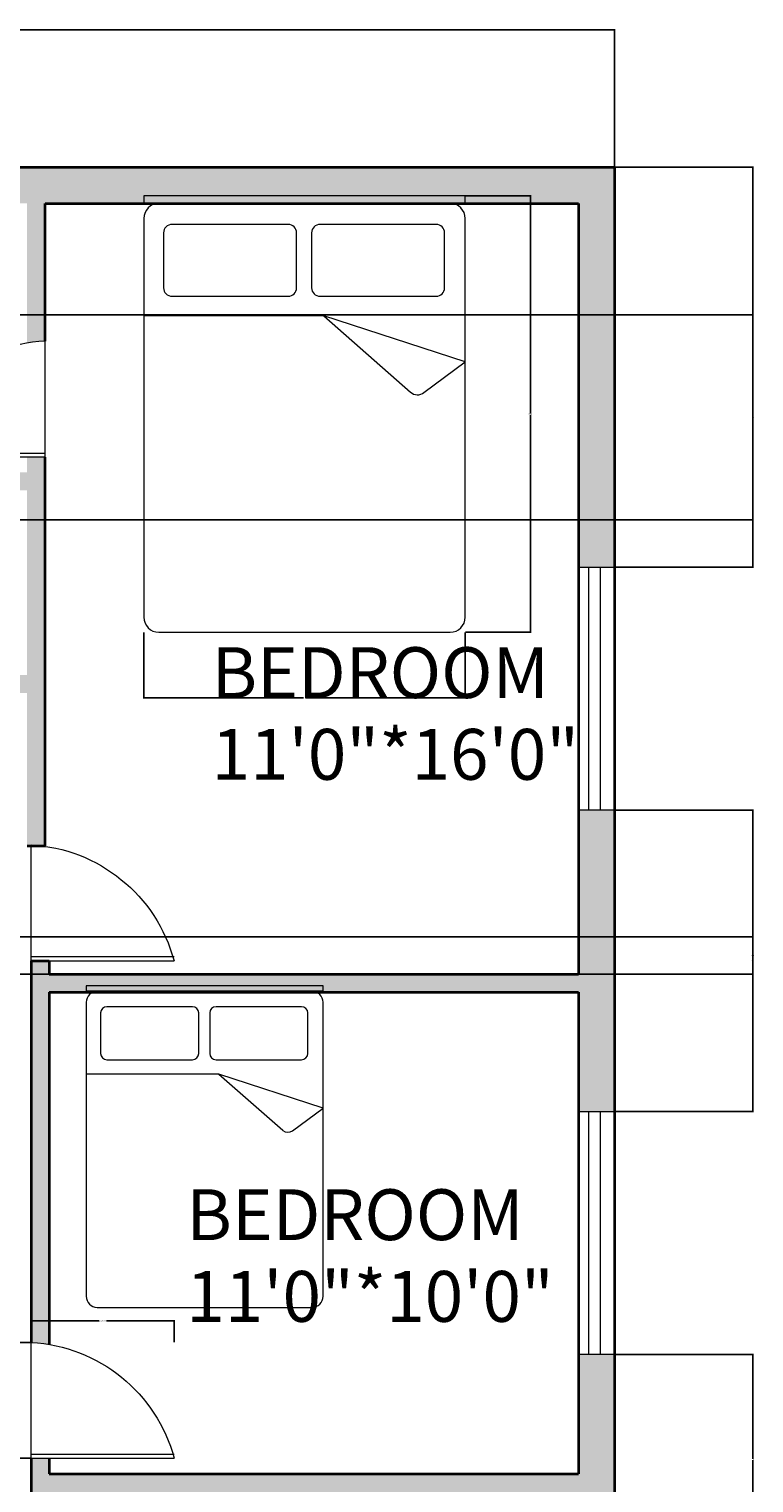
# Model space of a CAD drawing. Units: feet. Extents: x 2516 to 2945, y 1283 to 1993.
# Tile 3 of 3: x 2764 to 2945, y 1631 to 1993. Entities that reach past the tile are written whole.
import ezdxf

# ---------------------------------------------------------------- set-up
doc = ezdxf.new("R2010")
doc.units = ezdxf.units.FT
doc.layers.get('0').update_dxf_attribs({"lineweight": 18})
for name, color, linetype, lineweight in [('A-ANNO-DIMS', 2, 'Continuous', 18), ('A-AREA-IDEN', 7, 'Continuous', 18), ('A-FURN', 8, 'Continuous', 18), ('A-WALL', 7, 'Continuous', 35), ('A-WALL-PATT', 143, 'Continuous', 13), ('doors', 163, 'Continuous', 18), ('windows', 10, 'Continuous', 18)]:
    doc.layers.add(name, color=color, linetype=linetype, lineweight=lineweight)
doc.styles.get("Standard").update_dxf_attribs({"font": 'arial.ttf'})
doc.dimstyles.get("Standard").update_dxf_attribs({"dimtxt": 0.18, "dimasz": 0.18, "dimexe": 0.18, "dimexo": 0.0625, "dimgap": 0.09, "dimtad": 0, "dimtih": 1, "dimtoh": 1, "dimdec": 4, "dimzin": 0, "dimdsep": 46, "dimtxsty": 'Standard', "dimcen": 0.09, "dimadec": 0, "dimazin": 0, "dimtfac": 1, "dimtdec": 4, "dimtofl": 0, "dimtmove": 0, "dimatfit": 3, "dimfxl": 1, "dimtolj": 1, "dimtzin": 0, "dimarcsym": 0})

# ---------------------------------------------------------------- blocks, each defined once
blk = doc.blocks.new('door')
at = {"layer": 'doors'}
for p, q in [((-0.98, 0), (-0.98, 35.67)), ((0, 35.67), (0, 0)), ((-0.98, 0), (27.91, 0))]:
    blk.add_line(p, q, dxfattribs=at)
blk.add_arc((-11.23, -2.17), 39.2, 3.167, 74.8469, dxfattribs=at)
blk = doc.blocks.new('A$C164346CA')
for p, q in [((0, 2.035), (0, 2)), ((1.5, 2.035), (0, 2.035)), ((1.5, 2), (1.5, 2.035)), ((1.5, 2), (0, 2)), ((0, 1.93), (0, 0.07)), ((0.6731, 1.9024), (0.1319, 1.9024)), ((1.364, 1.9024), (0.8228, 1.9024)), ((1.5, 0.07), (1.5, 1.93)), ((0.0919, 1.8624), (0.0919, 1.6069)), ((0.7131, 1.6069), (0.7131, 1.8624)), ((0.7828, 1.8624), (0.7828, 1.6069)), ((1.404, 1.6069), (1.404, 1.8624)), ((0.1319, 1.5669), (0.6731, 1.5669)), ((0.8228, 1.5669), (1.364, 1.5669)), ((0.8395, 1.4761), (0, 1.4761)), ((0.8395, 1.4761), (1.2448, 1.12)), ((1.5, 1.2611), (0.8395, 1.4761)), ((1.3077, 1.1175), (1.5, 1.2611)), ((0.07, 0), (1.43, 0))]:
    blk.add_line(p, q)
for centre, radius, start, end in [((0.07, 1.93), 0.07, 90, 180), ((1.43, 1.93), 0.07, 0, 90), ((0.1319, 1.8624), 0.04, 90, 180), ((0.6731, 1.8624), 0.04, 0, 90), ((0.8228, 1.8624), 0.04, 90, 180), ((1.364, 1.8624), 0.04, 0, 90), ((0.1319, 1.6069), 0.04, 180, 270), ((0.6731, 1.6069), 0.04, 270, 0), ((0.8228, 1.6069), 0.04, 180, 270), ((1.364, 1.6069), 0.04, 270, 0), ((1.2778, 1.1575), 0.05, 228.69584, 306.75789), ((0.07, 0.07), 0.07, 180, 270), ((1.43, 0.07), 0.07, 270, 0)]:
    blk.add_arc(centre, radius, start, end)
blk = doc.blocks.new('WIN-STANDARD')
for p, q in [((2.52, 60.52), (2.52, 0)), ((5.4, 60.52), (5.4, 0))]:
    blk.add_line(p, q)
blk.add_lwpolyline([(0, 60.52), (9, 60.52), (9, 0), (0, 0)], close=True)
blk = doc.blocks.new('*D13')
at = {"layer": 'A-ANNO-DIMS', "color": 0, "lineweight": -2, "transparency": 16777216}
for p, q in [((2764.96, 1666.19), (2764.96, 1671.66)), ((2765.14, 1671.48), (2781.86, 1671.48)), ((2800.45, 1671.48), (2783.73, 1671.48)), ((2800.63, 1666.19), (2800.63, 1671.66))]:
    blk.add_line(p, q, dxfattribs=at)
at = {"layer": 'A-ANNO-DIMS', "color": 0, "transparency": 16777216}
for points in [[(2765.14, 1671.51), (2765.14, 1671.45), (2764.96, 1671.48)], [(2800.45, 1671.51), (2800.45, 1671.45), (2800.63, 1671.48)]]:
    blk.add_solid(points, dxfattribs=at)
at = {"layer": 'Defpoints', "color": 0, "transparency": 16777216}
for p in [(2800.63, 1671.48), (2764.96, 1666.13), (2800.63, 1666.13)]:
    blk.add_point(p, dxfattribs=at)
at = {"layer": 'A-ANNO-DIMS', "color": 0, "transparency": 16777216, "insert": (2782.79, 1671.48), "char_height": 0.18, "attachment_point": 5}
blk.add_mtext('\\A1;DOOR 36 TYP.', dxfattribs=at)
blk = doc.blocks.new('*D14')
at = {"layer": 'A-ANNO-DIMS', "color": 0, "lineweight": -2, "transparency": 16777216}
for p, q in [((2764.9, 1666.13), (2759.43, 1666.13)), ((2759.61, 1665.95), (2759.61, 1651.86)), ((2759.61, 1637.42), (2759.61, 1651.5)), ((2764.9, 1637.24), (2759.43, 1637.24))]:
    blk.add_line(p, q, dxfattribs=at)
at = {"layer": 'A-ANNO-DIMS', "color": 0, "transparency": 16777216}
for points in [[(2759.58, 1665.95), (2759.64, 1665.95), (2759.61, 1666.13)], [(2759.58, 1637.42), (2759.64, 1637.42), (2759.61, 1637.24)]]:
    blk.add_solid(points, dxfattribs=at)
at = {"layer": 'Defpoints', "color": 0, "transparency": 16777216}
for p in [(2759.61, 1666.13), (2764.96, 1666.13), (2764.96, 1637.24)]:
    blk.add_point(p, dxfattribs=at)
at = {"layer": 'A-ANNO-DIMS', "color": 0, "transparency": 16777216, "insert": (2759.61, 1651.68), "char_height": 0.18, "attachment_point": 5}
blk.add_mtext('\\A1;29 TYP.', dxfattribs=at)
blk = doc.blocks.new('*D15')
at = {"layer": 'A-ANNO-DIMS', "color": 0, "lineweight": -2, "transparency": 16777216}
for p, q in [((2873.22, 1951.73), (2889.64, 1951.73)), ((2889.46, 1951.55), (2889.46, 1897.56)), ((2889.46, 1843.21), (2889.46, 1897.2)), ((2873.22, 1843.03), (2889.64, 1843.03))]:
    blk.add_line(p, q, dxfattribs=at)
at = {"layer": 'A-ANNO-DIMS', "color": 0, "transparency": 16777216}
for points in [[(2889.43, 1951.55), (2889.49, 1951.55), (2889.46, 1951.73)], [(2889.43, 1843.21), (2889.49, 1843.21), (2889.46, 1843.03)]]:
    blk.add_solid(points, dxfattribs=at)
at = {"layer": 'Defpoints', "color": 0, "transparency": 16777216}
for p in [(2873.16, 1951.73), (2889.46, 1951.73), (2873.16, 1843.03)]:
    blk.add_point(p, dxfattribs=at)
at = {"layer": 'A-ANNO-DIMS', "color": 0, "transparency": 16777216, "insert": (2889.46, 1897.38), "char_height": 0.18, "attachment_point": 5}
blk.add_mtext('\\A1;BED 109', dxfattribs=at)
blk = doc.blocks.new('*D16')
at = {"layer": 'A-ANNO-DIMS', "color": 0, "lineweight": -2, "transparency": 16777216}
for p, q in [((2793.04, 1842.97), (2793.04, 1826.54)), ((2873.16, 1842.97), (2873.16, 1826.54)), ((2793.22, 1826.72), (2832.88, 1826.72)), ((2872.98, 1826.72), (2833.32, 1826.72))]:
    blk.add_line(p, q, dxfattribs=at)
at = {"layer": 'A-ANNO-DIMS', "color": 0, "transparency": 16777216}
for points in [[(2793.22, 1826.75), (2793.22, 1826.69), (2793.04, 1826.72)], [(2872.98, 1826.75), (2872.98, 1826.69), (2873.16, 1826.72)]]:
    blk.add_solid(points, dxfattribs=at)
at = {"layer": 'Defpoints', "color": 0, "transparency": 16777216}
for p in [(2793.04, 1843.03), (2873.16, 1843.03), (2873.16, 1826.72)]:
    blk.add_point(p, dxfattribs=at)
at = {"layer": 'A-ANNO-DIMS', "color": 0, "transparency": 16777216, "insert": (2833.1, 1826.72), "char_height": 0.18, "attachment_point": 5}
blk.add_mtext('\\A1;80', dxfattribs=at)
blk = doc.blocks.new('*D27')
at = {"layer": 'A-ANNO-DIMS', "color": 0, "lineweight": -2, "transparency": 16777216}
for p, q in [((2550.42, 1958.92), (2550.42, 1993.29)), ((2550.6, 1993.11), (2730.13, 1993.11)), ((2910.24, 1993.11), (2730.71, 1993.11)), ((2910.42, 1958.92), (2910.42, 1993.29))]:
    blk.add_line(p, q, dxfattribs=at)
at = {"layer": 'A-ANNO-DIMS', "color": 0, "transparency": 16777216}
for points in [[(2550.6, 1993.14), (2550.6, 1993.08), (2550.42, 1993.11)], [(2910.24, 1993.14), (2910.24, 1993.08), (2910.42, 1993.11)]]:
    blk.add_solid(points, dxfattribs=at)
at = {"layer": 'Defpoints', "color": 0, "transparency": 16777216}
for p in [(2910.42, 1993.11), (2550.42, 1958.86), (2910.42, 1958.86)]:
    blk.add_point(p, dxfattribs=at)
at = {"layer": 'A-ANNO-DIMS', "color": 0, "transparency": 16777216, "insert": (2730.42, 1993.11), "char_height": 0.18, "attachment_point": 5}
blk.add_mtext('\\A1;360', dxfattribs=at)
blk = doc.blocks.new('*D34')
at = {"layer": 'A-ANNO-DIMS', "color": 0, "lineweight": -2, "transparency": 16777216}
for p, q in [((2559.71, 1767.16), (2945.03, 1767.16)), ((2944.85, 1766.98), (2944.85, 1762.69)), ((2944.85, 1758.04), (2944.85, 1762.33)), ((2559.48, 1757.86), (2945.03, 1757.86))]:
    blk.add_line(p, q, dxfattribs=at)
at = {"layer": 'A-ANNO-DIMS', "color": 0, "transparency": 16777216}
for points in [[(2944.82, 1766.98), (2944.88, 1766.98), (2944.85, 1767.16)], [(2944.82, 1758.04), (2944.88, 1758.04), (2944.85, 1757.86)]]:
    blk.add_solid(points, dxfattribs=at)
at = {"layer": 'Defpoints', "color": 0, "transparency": 16777216}
for p in [(2559.64, 1767.16), (2944.85, 1767.16), (2559.42, 1757.86)]:
    blk.add_point(p, dxfattribs=at)
at = {"layer": 'A-ANNO-DIMS', "color": 0, "transparency": 16777216, "insert": (2944.85, 1762.51), "char_height": 0.18, "attachment_point": 5}
blk.add_mtext('\\A1;9.306', dxfattribs=at)
blk = doc.blocks.new('*D35')
at = {"layer": 'A-ANNO-DIMS', "color": 0, "lineweight": -2, "transparency": 16777216}
for p, q in [((2910.48, 1958.86), (2945.03, 1958.86)), ((2944.85, 1958.68), (2944.85, 1909.24)), ((2944.85, 1859.44), (2944.85, 1908.88)), ((2910.48, 1859.26), (2945.03, 1859.26))]:
    blk.add_line(p, q, dxfattribs=at)
at = {"layer": 'A-ANNO-DIMS', "color": 0, "transparency": 16777216}
for points in [[(2944.82, 1958.68), (2944.88, 1958.68), (2944.85, 1958.86)], [(2944.82, 1859.44), (2944.88, 1859.44), (2944.85, 1859.26)]]:
    blk.add_solid(points, dxfattribs=at)
at = {"layer": 'Defpoints', "color": 0, "transparency": 16777216}
for p in [(2910.42, 1958.86), (2944.85, 1958.86), (2910.42, 1859.26)]:
    blk.add_point(p, dxfattribs=at)
at = {"layer": 'A-ANNO-DIMS', "color": 0, "transparency": 16777216, "insert": (2944.85, 1909.06), "char_height": 0.18, "attachment_point": 5}
blk.add_mtext('\\A1;99.6', dxfattribs=at)
blk = doc.blocks.new('*D36')
at = {"layer": 'A-ANNO-DIMS', "color": 0, "lineweight": -2, "transparency": 16777216}
for p, q in [((2910.48, 1798.74), (2945.03, 1798.74)), ((2944.85, 1798.56), (2944.85, 1761.36)), ((2944.85, 1723.8), (2944.85, 1761)), ((2910.48, 1723.62), (2945.03, 1723.62))]:
    blk.add_line(p, q, dxfattribs=at)
at = {"layer": 'A-ANNO-DIMS', "color": 0, "transparency": 16777216}
for points in [[(2944.82, 1798.56), (2944.88, 1798.56), (2944.85, 1798.74)], [(2944.82, 1723.8), (2944.88, 1723.8), (2944.85, 1723.62)]]:
    blk.add_solid(points, dxfattribs=at)
at = {"layer": 'Defpoints', "color": 0, "transparency": 16777216}
for p in [(2910.42, 1798.74), (2944.85, 1798.74), (2910.42, 1723.62)]:
    blk.add_point(p, dxfattribs=at)
at = {"layer": 'A-ANNO-DIMS', "color": 0, "transparency": 16777216, "insert": (2944.85, 1761.18), "char_height": 0.18, "attachment_point": 5}
blk.add_mtext('\\A1;75.12', dxfattribs=at)
blk = doc.blocks.new('*D37')
at = {"layer": 'A-ANNO-DIMS', "color": 0, "lineweight": -2, "transparency": 16777216}
for p, q in [((2910.48, 1663.1), (2945.03, 1663.1)), ((2944.85, 1662.92), (2944.85, 1637.15)), ((2944.85, 1611.01), (2944.85, 1636.78)), ((2910.48, 1610.83), (2945.03, 1610.83))]:
    blk.add_line(p, q, dxfattribs=at)
at = {"layer": 'A-ANNO-DIMS', "color": 0, "transparency": 16777216}
for points in [[(2944.82, 1662.92), (2944.88, 1662.92), (2944.85, 1663.1)], [(2944.82, 1611.01), (2944.88, 1611.01), (2944.85, 1610.83)]]:
    blk.add_solid(points, dxfattribs=at)
at = {"layer": 'Defpoints', "color": 0, "transparency": 16777216}
for p in [(2910.42, 1663.1), (2944.85, 1663.1), (2910.42, 1610.83)]:
    blk.add_point(p, dxfattribs=at)
at = {"layer": 'A-ANNO-DIMS', "color": 0, "transparency": 16777216, "insert": (2944.85, 1636.97), "char_height": 0.18, "attachment_point": 5}
blk.add_mtext('\\A1;52.26', dxfattribs=at)
blk = doc.blocks.new('*D47')
at = {"layer": 'A-ANNO-DIMS', "color": 0, "lineweight": -2, "transparency": 16777216}
for p, q in [((2587.22, 1922.13), (2945.03, 1922.13)), ((2944.85, 1921.95), (2944.85, 1896.75)), ((2944.85, 1871.19), (2944.85, 1896.39)), ((2587.22, 1871.01), (2945.03, 1871.01))]:
    blk.add_line(p, q, dxfattribs=at)
at = {"layer": 'A-ANNO-DIMS', "color": 0, "transparency": 16777216}
for points in [[(2944.82, 1921.95), (2944.88, 1921.95), (2944.85, 1922.13)], [(2944.82, 1871.19), (2944.88, 1871.19), (2944.85, 1871.01)]]:
    blk.add_solid(points, dxfattribs=at)
at = {"layer": 'Defpoints', "color": 0, "transparency": 16777216}
for p in [(2587.15, 1922.13), (2587.15, 1871.01), (2944.85, 1871.01)]:
    blk.add_point(p, dxfattribs=at)
at = {"layer": 'A-ANNO-DIMS', "color": 0, "transparency": 16777216, "insert": (2944.85, 1896.57), "char_height": 0.18, "attachment_point": 5}
blk.add_mtext('\\A1;51.12', dxfattribs=at)

msp = doc.modelspace()

# ---------------------------------------------------------------- hatches: boundary and pattern name
at = {"layer": 'A-WALL-PATT'}
h = msp.add_hatch(color=256, dxfattribs=at)
h.dxf.hatch_style = 1
h.paths.add_polyline_path([(2763.9169, 1832.358), (2695.9169, 1832.358), (2695.9169, 1845.8137), (2691.4169, 1845.8137), (2691.4169, 1802.858), (2695.9169, 1802.858), (2695.9169, 1827.858), (2763.9169, 1827.858)])
h.paths.add_polyline_path([(2768.4169, 1886.6758), (2763.9169, 1886.6758), (2763.9169, 1789.8455), (2764.9169, 1789.8455), (2764.9169, 1790.0678, -0.01619533), (2767.4458, 1789.8455), (2768.4169, 1789.8455)])
h.paths.add_polyline_path([(2710.0911, 1958.858), (2663.1874, 1958.858), (2663.1874, 1949.858), (2691.4169, 1949.858), (2691.4169, 1878.358), (2763.9169, 1878.358), (2763.9169, 1882.858), (2695.9169, 1882.858), (2695.9169, 1949.858), (2710.0911, 1949.858)])
h.paths.add_polyline_path([(2910.4169, 1958.858), (2736.9631, 1958.858), (2736.9631, 1949.858), (2763.9169, 1949.858), (2763.9169, 1915.057, -0.02890868), (2768.4169, 1915.568), (2768.4169, 1949.858), (2901.4169, 1949.858), (2901.4169, 1859.2593), (2910.4169, 1859.2593)])
h.paths.add_polyline_path([(2910.4169, 1798.7389), (2901.4169, 1798.7389), (2901.4169, 1757.858), (2769.4169, 1757.858), (2769.4169, 1761.1755), (2764.9169, 1761.1755), (2764.9596, 1666.1291, -0.0286323), (2769.4169, 1665.6254), (2769.4169, 1753.358), (2901.4169, 1753.358), (2901.4169, 1723.6182), (2910.4169, 1723.6182)])
h.paths.add_polyline_path([(2910.4169, 1663.0978), (2901.4169, 1663.0978), (2901.4169, 1633.358), (2769.4169, 1633.358), (2769.4169, 1637.2369), (2764.9596, 1637.2369), (2764.9596, 1628.858), (2901.4169, 1628.858), (2901.4169, 1610.8331), (2910.4169, 1610.8331)])
h.paths.add_polyline_path([(2910.4169, 1572.5822), (2901.4169, 1572.5822), (2901.4169, 1552.858), (2812.9169, 1552.858), (2812.9169, 1548.358), (2817.4169, 1548.358), (2901.4169, 1548.358), (2901.4169, 1534.5783), (2910.4169, 1534.5783)])
h.paths.add_polyline_path([(2910.4169, 1507.7063), (2901.4169, 1507.7063), (2901.4169, 1500.358), (2817.4169, 1500.358), (2817.4169, 1518.131, -0.02890927), (2812.9169, 1517.6191), (2812.9169, 1500.358), (2803.3072, 1500.358, -0.02890868), (2802.7962, 1495.858), (2901.4169, 1495.858), (2901.4169, 1367.858), (2881.9751, 1367.858), (2881.9751, 1358.858), (2910.4169, 1358.858)])
h.paths.add_polyline_path([(2821.4547, 1367.858), (2769.4169, 1367.858), (2769.4169, 1495.858), (2774.415, 1495.858), (2774.415, 1500.358), (2760.4256, 1500.358), (2760.4256, 1495.858), (2764.9169, 1495.858), (2764.9169, 1367.858), (2764.9169, 1358.858), (2821.4547, 1358.858)])
h.paths.add_polyline_path([(2731.4104, 1499.858), (2559.4169, 1499.858), (2559.4169, 1495.358), (2731.4104, 1495.358)])
h.paths.add_polyline_path([(2559.4169, 1665.5276), (2550.4169, 1665.5276), (2550.4169, 1577.9069), (2559.4169, 1577.9069)])
h.paths.add_polyline_path([(2559.4169, 1767.1637), (2550.4169, 1767.1637), (2550.4169, 1726.0479), (2559.4169, 1726.0479)])
h.paths.add_polyline_path([(2695.9169, 1757.858), (2559.4169, 1757.858), (2559.4169, 1753.358), (2695.9169, 1753.358)])
h.paths.add_polyline_path([(2559.4169, 1949.858), (2602.667, 1949.858), (2602.667, 1958.858), (2550.4169, 1958.858), (2550.4169, 1827.6841), (2559.4169, 1827.6841)])

# ---------------------------------------------------------------- linework, layer by layer
at = {"layer": 'A-WALL'}
for p, q in [((2550.4169, 1958.858), (2910.4169, 1958.858)), ((2910.4169, 1958.858), (2910.4169, 1358.858)), ((2768.4169, 1949.858), (2901.4169, 1949.858)), ((2768.4169, 1915.568), (2768.4169, 1949.858)), ((2901.4169, 1949.858), (2901.4169, 1757.858)), ((2768.4169, 1789.8455), (2768.4169, 1886.6758)), ((2763.9169, 1789.8455), (2768.4169, 1789.8455)), ((2764.9169, 1761.1755), (2769.4169, 1761.1755)), ((2764.9169, 1761.1755), (2764.9596, 1666.1291)), ((2769.4169, 1761.1755), (2769.4169, 1757.858)), ((2769.4169, 1757.858), (2901.4169, 1757.858)), ((2769.4169, 1753.358), (2901.4169, 1753.358)), ((2769.4169, 1753.358), (2769.4169, 1665.6254)), ((2901.4169, 1753.358), (2901.4169, 1633.358)), ((2764.9596, 1637.2369), (2764.9596, 1628.858)), ((2769.4169, 1637.2369), (2769.4169, 1633.358)), ((2769.4169, 1633.358), (2901.4169, 1633.358))]:
    msp.add_line(p, q, dxfattribs=at)

# ---------------------------------------------------------------- block references
at = {"layer": 'A-FURN'}
for p, xscale, yscale, zscale in [((2793.0365, 1843.0276), 53.41517557031528, 53.41517557031528, 53.41517557031528), ((2778.6489, 1674.8478), 39.37235568073177, 39.37235568073177, 39.37235568073177)]:
    msp.add_blockref('A$C164346CA', p, dxfattribs=dict(at, xscale=xscale, yscale=yscale, zscale=zscale))
at = {"layer": 'doors', "rotation": 89.99999999999999}
msp.add_blockref('door', (2768.4169, 1887.6584), dxfattribs=at)
at = {"layer": 'doors', "xscale": -1, "rotation": 270}
for p in [(2764.9169, 1762.1581), (2764.9596, 1638.2195)]:
    msp.add_blockref('door', p, dxfattribs=at)
at = {"layer": 'windows'}
for p in [(2901.417, 1798.7394), (2901.417, 1663.0982)]:
    msp.add_blockref('WIN-STANDARD', p, dxfattribs=at)

# ---------------------------------------------------------------- texts
at = {"layer": 'A-AREA-IDEN'}
for s, height, p in [('BEDROOM', 12.66946, (2809.9355, 1826.6319)), ('11\'0"*16\'0"', 12.669464, (2809.9355, 1806.2795)), ('BEDROOM', 12.66946, (2803.6284, 1691.5908)), ('11\'0"*10\'0"', 12.669464, (2803.6284, 1671.2384))]:
    msp.add_text(s, height=height, dxfattribs=at).set_placement(p)

# ---------------------------------------------------------------- dimensions: what is measured, and where the dimension line sits
at = {"layer": 'A-ANNO-DIMS'}
for base, p1, p2, picture, middle in [((2910.4169, 1993.108), (2550.4169, 1958.858), (2910.4169, 1958.858), '*D27', (2730.4169, 1993.108)), ((2873.1593, 1826.7227), (2793.0365, 1843.0276), (2873.1593, 1843.0276), '*D16', (2833.0979, 1826.7227))]:
    dim = msp.add_linear_dim(base=base, p1=p1, p2=p2, dimstyle='Standard', override={"dimdec": 0, "dimlfac": 1, "dimrnd": 0, "dimzin": 0, "dimdsep": 46, "dimlunit": 2}, dxfattribs=at)
    dim.commit()
    dim.dimension.update_dxf_attribs({"geometry": picture, "text_midpoint": middle})
for base, p1, p2, override, picture, middle in [((2944.8487, 1958.858), (2910.4169, 1859.2593), (2910.4169, 1958.858), {"dimdec": 1, "dimlfac": 1, "dimrnd": 0, "dimzin": 0, "dimdsep": 46, "dimlunit": 2}, '*D35', (2944.8487, 1909.0587)), ((2944.8487, 1871.0142), (2587.155, 1922.1312), (2587.155, 1871.0142), {"dimdec": 2, "dimlfac": 1, "dimrnd": 0, "dimzin": 0, "dimdsep": 46, "dimlunit": 2}, '*D47', (2944.8487, 1896.5727)), ((2944.8487, 1798.7389), (2910.4169, 1723.6182), (2910.4169, 1798.7389), {"dimdec": 2, "dimlfac": 1, "dimrnd": 0, "dimzin": 0, "dimdsep": 46, "dimlunit": 2}, '*D36', (2944.8487, 1761.1786)), ((2944.8487, 1767.1637), (2559.4169, 1757.858), (2559.6429, 1767.1637), {"dimdec": 3, "dimlfac": 1, "dimrnd": 0, "dimzin": 0, "dimdsep": 46, "dimlunit": 2}, '*D34', (2944.8487, 1762.5109)), ((2944.8487, 1663.0978), (2910.4169, 1610.8331), (2910.4169, 1663.0978), {"dimdec": 2, "dimlfac": 1, "dimrnd": 0, "dimzin": 0, "dimdsep": 46, "dimlunit": 2}, '*D37', (2944.8487, 1636.9654))]:
    dim = msp.add_linear_dim(base=base, p1=p1, p2=p2, angle=90, dimstyle='Standard', override=override, dxfattribs=at)
    dim.commit()
    dim.dimension.update_dxf_attribs({"geometry": picture, "text_midpoint": middle})
for base, p1, p2, text, picture, middle in [((2889.4643, 1951.7275), (2873.1593, 1843.0276), (2873.1593, 1951.7275), 'BED <>', '*D15', (2889.4643, 1897.3776)), ((2759.6091, 1666.1291), (2764.9596, 1637.2369), (2764.9596, 1666.1291), '<> TYP.', '*D14', (2759.6091, 1651.683))]:
    dim = msp.add_linear_dim(base=base, p1=p1, p2=p2, angle=90, text=text, dimstyle='Standard', override={"dimdec": 0, "dimlfac": 1, "dimrnd": 0, "dimzin": 0, "dimdsep": 46, "dimlunit": 2}, dxfattribs=at)
    dim.commit()
    dim.dimension.update_dxf_attribs({"geometry": picture, "text_midpoint": middle})
dim = msp.add_linear_dim(base=(2800.6296, 1671.4796), p1=(2764.9596, 1666.1291), p2=(2800.6296, 1666.1291), text='DOOR <> TYP.', dimstyle='Standard', override={"dimdec": 0, "dimlfac": 1, "dimrnd": 0, "dimzin": 0, "dimdsep": 46, "dimlunit": 2}, dxfattribs=at)
dim.commit()
dim.dimension.update_dxf_attribs({"geometry": '*D13', "text_midpoint": (2782.7946, 1671.4796)})

doc.saveas('drawing.dxf')
